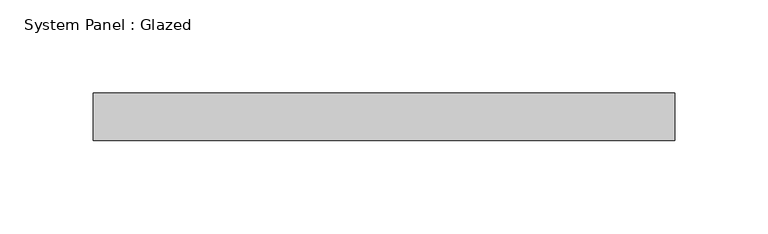
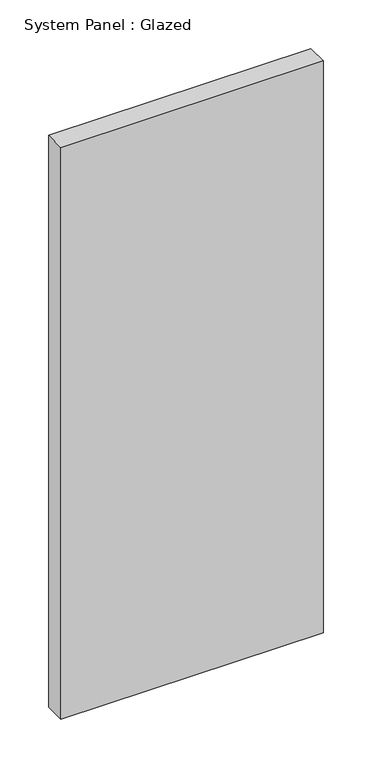
"""IFC4 building model written with IfcOpenShell, lengths in millimetres: plate geometry, System Panel : Glazed."""

from ifc_helpers import new_model, si_unit, origin, origin_with_axes, place, context, project, spatial, polyline, outline, extrude, source, transform, mapped, element, save


def system_panel_glazed_6328bcbd(model_context):
    return source(origin(), model_context, "Body", "SweptSolid", [
        extrude(outline(polyline([(155.575, 19.05), (-155.575, 19.05), (-155.575, 44.45), (155.575, 44.45), (155.575, 19.05)])), origin_with_axes(), (0.0, 0.0, 1.0), 717.55),
    ])


if __name__ == "__main__":
    model = new_model("IFC4")
    model_context = context("Model", 3, world=origin())
    ifc_project = project(units=[si_unit("LENGTHUNIT", "METRE", prefix="MILLI")], contexts=[model_context])
    site = spatial("IfcSite", under=ifc_project)
    building = spatial("IfcBuilding", under=site)
    placement = place(None, origin())
    system_panel_glazed_shape = system_panel_glazed_6328bcbd(model_context)
    element("IfcPlate", 1, ObjectType="System Panel : Glazed", at=placement, inside=building, context=model_context, shape_type="MappedRepresentation", body=[
        mapped(system_panel_glazed_shape, transform((0.0, 0.0, 0.0), x_axis=(1.0, 0.0, 0.0), y_axis=(0.0, 1.0, 0.0), z_axis=(0.0, 0.0, 1.0))),
    ])
    save(model, "model.ifc")

# Revit data of these elements
# Type "System Panel : Glazed"
#   Construction Type Id = "GSP4R"
#   Analytic Construction = "1/8 in Pilkington single glazing"
#   Visual Light Transmittance = 0.9
#   Solar Heat Gain Coefficient = 0.86
#   Heat Transfer Coefficient (U) = 1.18115 BTU/(h·ft²·°F)
# Element 1 (IfcPlate, "System Panel : Glazed")
#   Materials on its faces: "Glass"
# Materials
#   "Glass": class "Glass", colour RGB 0 128 192, transparency 0.75, Description = "Soda Lime Glass", Cost = 0
